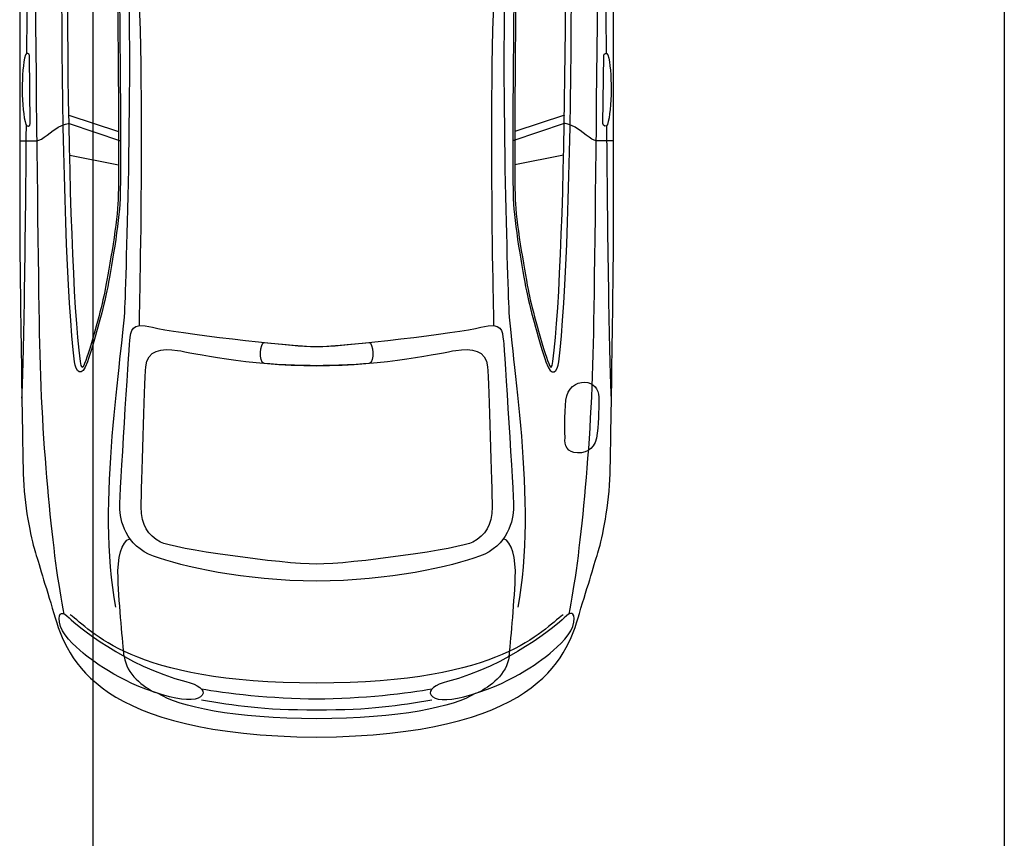
# Model space of a CAD drawing. Units: inches. Extents: x 1863 to 2938, y 1238 to 2492.
# Tile 3 of 12: x 2219 to 2283, y 1345 to 1398. Entities that reach past the tile are written whole.
import ezdxf

# ---------------------------------------------------------------- set-up
doc = ezdxf.new("R2010")
doc.units = ezdxf.units.IN
doc.layers.add('A-ANNO-DIMS', color=2, linetype='Continuous', lineweight=18)
doc.layers.add('AUDI', color=7, linetype='Continuous', lineweight=25)
doc.styles.get("Standard").update_dxf_attribs({"font": 'arial.ttf'})
doc.dimstyles.new('ISO-25', dxfattribs={"dimtxt": 7, "dimasz": 2.5, "dimexe": 1.25, "dimexo": 0.625, "dimtad": 1, "dimdec": 0, "dimlunit": 3, "dimtxsty": 'Standard', "dimcen": 2.5, "dimadec": 0, "dimazin": 0, "dimtfac": 1, "dimtdec": 0, "dimtmove": 0, "dimatfit": 3, "dimfxl": 1, "dimarcsym": 0})

# ---------------------------------------------------------------- blocks, each defined once
blk = doc.blocks.new('*D58')
at = {"layer": 'A-ANNO-DIMS', "color": 0, "lineweight": -2, "transparency": 16777216}
for p, q in [((2283.384, 1624.448), (2283.384, 1243.072)), ((2223.915, 1623.598), (2223.915, 1243.072)), ((2226.415, 1244.322), (2280.884, 1244.322))]:
    blk.add_line(p, q, dxfattribs=at)
at = {"layer": 'A-ANNO-DIMS', "color": 0, "transparency": 16777216}
for points in [[(2226.415, 1244.739), (2226.415, 1243.905), (2223.915, 1244.322)], [(2280.884, 1244.739), (2280.884, 1243.905), (2283.384, 1244.322)]]:
    blk.add_solid(points, dxfattribs=at)
at = {"layer": 'Defpoints', "color": 0, "transparency": 16777216}
for p in [(2283.384, 1625.073), (2223.915, 1624.223), (2283.384, 1244.322)]:
    blk.add_point(p, dxfattribs=at)
at = {"layer": 'A-ANNO-DIMS', "color": 0, "transparency": 16777216, "insert": (2253.65, 1248.566), "char_height": 7, "attachment_point": 5}
blk.add_mtext('4\'-11 1/2"', dxfattribs=at)

msp = doc.modelspace()

# ---------------------------------------------------------------- linework, layer by layer
at = {"layer": 'AUDI'}
for points, knots in [([(2238.512, 1351.601), (2224.304, 1351.757), (2222.24, 1356.535), (2221.369, 1359.683), (2221.369, 1359.683), (2220.8, 1361.542), (2220.345, 1363.021), (2220.118, 1363.779), (2220.118, 1363.779), (2219.89, 1364.538), (2219.398, 1366.852), (2219.359, 1368.786), (2219.359, 1368.786), (2219.321, 1370.721), (2219.134, 1382.255), (2219.134, 1385.438), (2219.134, 1385.438), (2219.134, 1388.621), (2219.134, 1403.534), (2219.134, 1405.655), (2219.134, 1405.655), (2219.134, 1407.776), (2219.587, 1416.238), (2219.587, 1418.931), (2219.587, 1418.931), (2219.587, 1421.624), (2219.134, 1425.003), (2219.134, 1426.403), (2219.134, 1426.403), (2219.134, 1427.803), (2219.397, 1435.203), (2219.511, 1436.834), (2219.511, 1436.834), (2219.625, 1438.465), (2220.236, 1439.39), (2220.762, 1440.551), (2220.762, 1440.551), (2222.809, 1445.064), (2228.041, 1447.53), (2228.61, 1447.909), (2228.61, 1447.909), (2229.178, 1448.289), (2229.782, 1448.495), (2230.505, 1448.495), (2230.505, 1448.495), (2231.228, 1448.495), (2231.415, 1448.137), (2231.718, 1448.213), (2231.718, 1448.213), (2232.021, 1448.289), (2232.777, 1448.495), (2233.614, 1448.495), (2233.614, 1448.495), (2234.451, 1448.495), (2238.512, 1448.495), (2238.512, 1448.495), (2238.512, 1448.495), (2238.512, 1448.495), (2242.574, 1448.495), (2243.411, 1448.495), (2243.411, 1448.495), (2244.248, 1448.495), (2245.003, 1448.289), (2245.306, 1448.213), (2245.306, 1448.213), (2245.61, 1448.137), (2245.796, 1448.495), (2246.52, 1448.495), (2246.52, 1448.495), (2247.243, 1448.495), (2247.846, 1448.289), (2248.415, 1447.909), (2248.415, 1447.909), (2248.984, 1447.53), (2254.215, 1445.064), (2256.262, 1440.551), (2256.262, 1440.551), (2256.789, 1439.39), (2257.4, 1438.465), (2257.513, 1436.834), (2257.513, 1436.834), (2257.627, 1435.203), (2257.891, 1427.803), (2257.891, 1426.403), (2257.891, 1426.403), (2257.891, 1425.003), (2257.438, 1421.624), (2257.438, 1418.931), (2257.438, 1418.931), (2257.438, 1416.238), (2257.891, 1407.776), (2257.891, 1405.655), (2257.891, 1405.655), (2257.891, 1403.534), (2257.891, 1388.621), (2257.891, 1385.438), (2257.891, 1385.438), (2257.891, 1382.255), (2257.703, 1370.721), (2257.665, 1368.786), (2257.665, 1368.786), (2257.627, 1366.852), (2257.134, 1364.538), (2256.907, 1363.779), (2256.907, 1363.779), (2256.679, 1363.021), (2256.225, 1361.541), (2255.656, 1359.683), (2255.656, 1359.683), (2254.784, 1356.535), (2252.721, 1351.757), (2238.512, 1351.601)], [0, 0, 0, 0, 0.035714, 0.035714, 0.035714, 0.035714, 0.071429, 0.071429, 0.071429, 0.071429, 0.107143, 0.107143, 0.107143, 0.107143, 0.142857, 0.142857, 0.142857, 0.142857, 0.178571, 0.178571, 0.178571, 0.178571, 0.214286, 0.214286, 0.214286, 0.214286, 0.25, 0.25, 0.25, 0.25, 0.285714, 0.285714, 0.285714, 0.285714, 0.321429, 0.321429, 0.321429, 0.321429, 0.357143, 0.357143, 0.357143, 0.357143, 0.392857, 0.392857, 0.392857, 0.392857, 0.428571, 0.428571, 0.428571, 0.428571, 0.464286, 0.464286, 0.464286, 0.464286, 0.5, 0.5, 0.5, 0.5, 0.535714, 0.535714, 0.535714, 0.535714, 0.571429, 0.571429, 0.571429, 0.571429, 0.607143, 0.607143, 0.607143, 0.607143, 0.642857, 0.642857, 0.642857, 0.642857, 0.678571, 0.678571, 0.678571, 0.678571, 0.714286, 0.714286, 0.714286, 0.714286, 0.75, 0.75, 0.75, 0.75, 0.785714, 0.785714, 0.785714, 0.785714, 0.821429, 0.821429, 0.821429, 0.821429, 0.857143, 0.857143, 0.857143, 0.857143, 0.892857, 0.892857, 0.892857, 0.892857, 0.928571, 0.928571, 0.928571, 0.928571, 0.964286, 0.964286, 0.964286, 0.964286, 1, 1, 1, 1]), ([(2222.035, 1359.641), (2221.321, 1363.213), (2220.561, 1370.446), (2220.431, 1377.979), (2220.431, 1377.979), (2220.301, 1385.512), (2219.977, 1414.474), (2220.172, 1420.578), (2220.172, 1420.578), (2220.366, 1426.682), (2220.475, 1434.382), (2221.557, 1439.624)], [0, 0, 0, 0, 0.333333, 0.333333, 0.333333, 0.333333, 0.666667, 0.666667, 0.666667, 0.666667, 1, 1, 1, 1]), ([(2254.99, 1359.641), (2255.704, 1363.213), (2256.464, 1370.446), (2256.593, 1377.979), (2256.593, 1377.979), (2256.723, 1385.512), (2257.048, 1414.474), (2256.853, 1420.578), (2256.853, 1420.578), (2256.658, 1426.682), (2256.549, 1434.382), (2255.468, 1439.624)], [0, 0, 0, 0, 0.333333, 0.333333, 0.333333, 0.333333, 0.666667, 0.666667, 0.666667, 0.666667, 1, 1, 1, 1]), ([(2222.717, 1376.103), (2222.793, 1375.509), (2223.16, 1374.97), (2223.554, 1376.103), (2223.554, 1376.103), (2223.947, 1377.235), (2224.587, 1379.549), (2224.784, 1380.534), (2224.784, 1380.534), (2224.981, 1381.519), (2225.572, 1384.768), (2225.67, 1386.393), (2225.67, 1386.393), (2225.768, 1388.018), (2225.67, 1396.339), (2225.67, 1398.308), (2225.67, 1398.308), (2225.67, 1400.278), (2224.833, 1407.024), (2224.538, 1408.648), (2224.538, 1408.648), (2224.243, 1410.273), (2223.603, 1413.523), (2222.371, 1417.183), (2222.371, 1417.183), (2221.635, 1413.129), (2221.733, 1383.833), (2222.717, 1376.103)], [0, 0, 0, 0, 0.142857, 0.142857, 0.142857, 0.142857, 0.285714, 0.285714, 0.285714, 0.285714, 0.428571, 0.428571, 0.428571, 0.428571, 0.571429, 0.571429, 0.571429, 0.571429, 0.714286, 0.714286, 0.714286, 0.714286, 0.857143, 0.857143, 0.857143, 0.857143, 1, 1, 1, 1]), ([(2254.308, 1376.103), (2254.232, 1375.509), (2253.864, 1374.97), (2253.471, 1376.103), (2253.471, 1376.103), (2253.077, 1377.235), (2252.437, 1379.549), (2252.241, 1380.534), (2252.241, 1380.534), (2252.044, 1381.519), (2251.453, 1384.768), (2251.355, 1386.393), (2251.355, 1386.393), (2251.256, 1388.018), (2251.355, 1396.339), (2251.355, 1398.308), (2251.355, 1398.308), (2251.355, 1400.278), (2252.191, 1407.024), (2252.487, 1408.648), (2252.487, 1408.648), (2252.782, 1410.273), (2253.422, 1413.523), (2254.654, 1417.183), (2254.654, 1417.183), (2255.39, 1413.129), (2255.292, 1383.833), (2254.308, 1376.103)], [0, 0, 0, 0, 0.142857, 0.142857, 0.142857, 0.142857, 0.285714, 0.285714, 0.285714, 0.285714, 0.428571, 0.428571, 0.428571, 0.428571, 0.571429, 0.571429, 0.571429, 0.571429, 0.714286, 0.714286, 0.714286, 0.714286, 0.857143, 0.857143, 0.857143, 0.857143, 1, 1, 1, 1]), ([(2223.091, 1376.134), (2223.091, 1376.134), (2223.091, 1376.134), (2223.091, 1376.134), (2223.091, 1376.134), (2223.119, 1375.917), (2223.178, 1375.791), (2223.221, 1375.73), (2223.221, 1375.73), (2223.266, 1375.783), (2223.344, 1375.902), (2223.442, 1376.185), (2223.442, 1376.185), (2223.826, 1377.289), (2224.465, 1379.591), (2224.663, 1380.583), (2224.663, 1380.583), (2224.901, 1381.772), (2225.453, 1384.89), (2225.545, 1386.408), (2225.545, 1386.408), (2225.617, 1387.597), (2225.582, 1392.452), (2225.559, 1395.665), (2225.559, 1395.665), (2225.559, 1395.665), (2225.544, 1398.309), (2225.544, 1398.309), (2225.544, 1398.309), (2225.544, 1400.273), (2224.699, 1407.05), (2224.417, 1408.603), (2224.417, 1408.603), (2223.944, 1411.2), (2223.332, 1413.673), (2222.608, 1415.993), (2222.608, 1415.993), (2222.029, 1409.274), (2222.179, 1383.297), (2223.091, 1376.134)], [0, 0, 0, 0, 0.1, 0.1, 0.1, 0.1, 0.2, 0.2, 0.2, 0.2, 0.3, 0.3, 0.3, 0.3, 0.4, 0.4, 0.4, 0.4, 0.5, 0.5, 0.5, 0.5, 0.6, 0.6, 0.6, 0.6, 0.7, 0.7, 0.7, 0.7, 0.8, 0.8, 0.8, 0.8, 0.9, 0.9, 0.9, 0.9, 1, 1, 1, 1]), ([(2253.933, 1376.134), (2253.933, 1376.134), (2253.933, 1376.134), (2253.933, 1376.134), (2253.933, 1376.134), (2253.906, 1375.917), (2253.846, 1375.791), (2253.804, 1375.73), (2253.804, 1375.73), (2253.759, 1375.783), (2253.681, 1375.902), (2253.582, 1376.185), (2253.582, 1376.185), (2253.199, 1377.289), (2252.56, 1379.591), (2252.361, 1380.583), (2252.361, 1380.583), (2252.124, 1381.772), (2251.572, 1384.89), (2251.48, 1386.408), (2251.48, 1386.408), (2251.408, 1387.597), (2251.442, 1392.452), (2251.465, 1395.665), (2251.465, 1395.665), (2251.465, 1395.665), (2251.48, 1398.309), (2251.48, 1398.309), (2251.48, 1398.309), (2251.48, 1400.273), (2252.326, 1407.05), (2252.608, 1408.603), (2252.608, 1408.603), (2253.08, 1411.2), (2253.692, 1413.673), (2254.417, 1415.993), (2254.417, 1415.993), (2254.995, 1409.274), (2254.846, 1383.297), (2253.933, 1376.134)], [0, 0, 0, 0, 0.1, 0.1, 0.1, 0.1, 0.2, 0.2, 0.2, 0.2, 0.3, 0.3, 0.3, 0.3, 0.4, 0.4, 0.4, 0.4, 0.5, 0.5, 0.5, 0.5, 0.6, 0.6, 0.6, 0.6, 0.7, 0.7, 0.7, 0.7, 0.8, 0.8, 0.8, 0.8, 0.9, 0.9, 0.9, 0.9, 1, 1, 1, 1]), ([(2226.062, 1406.214), (2226.571, 1397.024), (2226.092, 1382.572), (2225.981, 1379.639), (2225.981, 1379.639), (2225.87, 1376.706), (2224.075, 1366.744), (2225.391, 1360.079)], [0, 0, 0, 0, 0.5, 0.5, 0.5, 0.5, 1, 1, 1, 1]), ([(2250.963, 1406.214), (2250.454, 1397.024), (2250.933, 1382.572), (2251.044, 1379.639), (2251.044, 1379.639), (2251.154, 1376.706), (2252.949, 1366.744), (2251.634, 1360.079)], [0, 0, 0, 0, 0.5, 0.5, 0.5, 0.5, 1, 1, 1, 1]), ([(2219.828, 1391.652), (2219.828, 1391.478), (2219.591, 1391.413), (2219.538, 1391.587), (2219.538, 1391.587), (2219.379, 1392.086), (2219.301, 1392.976), (2219.301, 1393.866), (2219.301, 1393.866), (2219.301, 1394.757), (2219.353, 1395.625), (2219.511, 1396.146), (2219.511, 1396.146), (2219.564, 1396.298), (2219.775, 1396.255), (2219.775, 1396.081), (2219.775, 1396.081), (2219.775, 1396.081), (2219.828, 1391.652), (2219.828, 1391.652)], [0, 0, 0, 0, 0.2, 0.2, 0.2, 0.2, 0.4, 0.4, 0.4, 0.4, 0.6, 0.6, 0.6, 0.6, 0.8, 0.8, 0.8, 0.8, 1, 1, 1, 1]), ([(2257.196, 1391.652), (2257.196, 1391.478), (2257.434, 1391.413), (2257.487, 1391.587), (2257.487, 1391.587), (2257.645, 1392.086), (2257.724, 1392.976), (2257.724, 1393.866), (2257.724, 1393.866), (2257.724, 1394.757), (2257.671, 1395.625), (2257.513, 1396.146), (2257.513, 1396.146), (2257.46, 1396.298), (2257.25, 1396.255), (2257.25, 1396.081), (2257.25, 1396.081), (2257.25, 1396.081), (2257.196, 1391.652), (2257.196, 1391.652)], [0, 0, 0, 0, 0.2, 0.2, 0.2, 0.2, 0.4, 0.4, 0.4, 0.4, 0.6, 0.6, 0.6, 0.6, 0.8, 0.8, 0.8, 0.8, 1, 1, 1, 1]), ([(2219.134, 1390.537), (2219.134, 1390.537), (2219.988, 1390.537), (2220.268, 1390.537), (2220.268, 1390.537), (2220.548, 1390.537), (2221.292, 1391.217), (2221.635, 1391.415), (2221.635, 1391.415), (2221.977, 1391.614), (2222.354, 1391.661), (2222.354, 1391.661)], [0, 0, 0, 0, 0.333333, 0.333333, 0.333333, 0.333333, 0.666667, 0.666667, 0.666667, 0.666667, 1, 1, 1, 1]), ([(2257.891, 1390.537), (2257.891, 1390.537), (2257.037, 1390.537), (2256.757, 1390.537), (2256.757, 1390.537), (2256.476, 1390.537), (2255.733, 1391.217), (2255.39, 1391.415), (2255.39, 1391.415), (2255.047, 1391.614), (2254.671, 1391.661), (2254.671, 1391.661)], [0, 0, 0, 0, 0.333333, 0.333333, 0.333333, 0.333333, 0.666667, 0.666667, 0.666667, 0.666667, 1, 1, 1, 1]), ([(2238.512, 1361.794), (2243.289, 1361.794), (2247.305, 1362.753), (2249.149, 1363.417), (2249.149, 1363.417), (2250.992, 1364.081), (2251.361, 1365.778), (2251.361, 1366.627), (2251.361, 1366.627), (2251.361, 1367.475), (2250.771, 1376.809), (2250.697, 1377.473), (2250.697, 1377.473), (2250.624, 1378.137), (2250.66, 1378.728), (2249.222, 1378.359), (2249.222, 1378.359), (2247.784, 1377.99), (2240.299, 1377.104), (2238.512, 1377.104), (2238.512, 1377.104), (2236.726, 1377.105), (2229.24, 1377.99), (2227.802, 1378.359), (2227.802, 1378.359), (2226.364, 1378.728), (2226.401, 1378.137), (2226.327, 1377.473), (2226.327, 1377.473), (2226.254, 1376.809), (2225.664, 1367.475), (2225.664, 1366.627), (2225.664, 1366.627), (2225.664, 1365.778), (2226.032, 1364.081), (2227.876, 1363.417), (2227.876, 1363.417), (2229.72, 1362.753), (2233.735, 1361.794), (2238.512, 1361.794)], [0, 0, 0, 0, 0.1, 0.1, 0.1, 0.1, 0.2, 0.2, 0.2, 0.2, 0.3, 0.3, 0.3, 0.3, 0.4, 0.4, 0.4, 0.4, 0.5, 0.5, 0.5, 0.5, 0.6, 0.6, 0.6, 0.6, 0.7, 0.7, 0.7, 0.7, 0.8, 0.8, 0.8, 0.8, 0.9, 0.9, 0.9, 0.9, 1, 1, 1, 1]), ([(2238.512, 1361.794), (2243.289, 1361.794), (2247.305, 1362.753), (2249.149, 1363.417), (2249.149, 1363.417), (2250.992, 1364.081), (2251.361, 1365.778), (2251.361, 1366.627), (2251.361, 1366.627), (2251.361, 1367.475), (2250.771, 1376.809), (2250.697, 1377.473), (2250.697, 1377.473), (2250.624, 1378.137), (2250.66, 1378.728), (2249.222, 1378.359), (2249.222, 1378.359), (2247.784, 1377.99), (2240.299, 1377.104), (2238.512, 1377.104), (2238.512, 1377.104), (2236.726, 1377.104), (2229.24, 1377.99), (2227.802, 1378.359), (2227.802, 1378.359), (2226.364, 1378.728), (2226.401, 1378.137), (2226.327, 1377.473), (2226.327, 1377.473), (2226.254, 1376.809), (2225.664, 1367.475), (2225.664, 1366.627), (2225.664, 1366.627), (2225.664, 1365.778), (2226.032, 1364.081), (2227.876, 1363.417), (2227.876, 1363.417), (2229.72, 1362.753), (2233.735, 1361.794), (2238.512, 1361.794)], [0, 0, 0, 0, 0.1, 0.1, 0.1, 0.1, 0.2, 0.2, 0.2, 0.2, 0.3, 0.3, 0.3, 0.3, 0.4, 0.4, 0.4, 0.4, 0.5, 0.5, 0.5, 0.5, 0.6, 0.6, 0.6, 0.6, 0.7, 0.7, 0.7, 0.7, 0.8, 0.8, 0.8, 0.8, 0.9, 0.9, 0.9, 0.9, 1, 1, 1, 1]), ([(2238.512, 1362.898), (2240.778, 1362.898), (2247.895, 1363.897), (2248.706, 1364.339), (2248.706, 1364.339), (2249.517, 1364.782), (2249.96, 1365.409), (2249.96, 1366.627), (2249.96, 1366.627), (2249.96, 1367.844), (2249.738, 1374.67), (2249.665, 1375.776), (2249.665, 1375.776), (2249.591, 1376.883), (2248.595, 1376.994), (2247.6, 1376.846), (2247.6, 1376.846), (2246.604, 1376.699), (2243.101, 1375.85), (2238.512, 1375.85), (2238.512, 1375.85), (2233.923, 1375.85), (2230.42, 1376.699), (2229.425, 1376.846), (2229.425, 1376.846), (2228.429, 1376.994), (2227.434, 1376.883), (2227.36, 1375.776), (2227.36, 1375.776), (2227.286, 1374.67), (2227.065, 1367.844), (2227.065, 1366.627), (2227.065, 1366.627), (2227.065, 1365.409), (2227.507, 1364.782), (2228.318, 1364.339), (2228.318, 1364.339), (2229.13, 1363.897), (2236.246, 1362.898), (2238.512, 1362.898)], [0, 0, 0, 0, 0.1, 0.1, 0.1, 0.1, 0.2, 0.2, 0.2, 0.2, 0.3, 0.3, 0.3, 0.3, 0.4, 0.4, 0.4, 0.4, 0.5, 0.5, 0.5, 0.5, 0.6, 0.6, 0.6, 0.6, 0.7, 0.7, 0.7, 0.7, 0.8, 0.8, 0.8, 0.8, 0.9, 0.9, 0.9, 0.9, 1, 1, 1, 1]), ([(2238.512, 1375.85), (2238.512, 1375.85), (2241.218, 1375.898), (2241.924, 1376.002), (2241.924, 1376.002), (2242.365, 1376.067), (2242.157, 1377.387), (2241.951, 1377.367), (2241.951, 1377.367), (2240.654, 1377.241), (2239.564, 1377.104), (2238.512, 1377.104), (2238.512, 1377.104), (2237.46, 1377.104), (2236.37, 1377.241), (2235.074, 1377.367), (2235.074, 1377.367), (2234.867, 1377.387), (2234.66, 1376.067), (2235.101, 1376.002), (2235.101, 1376.002), (2235.807, 1375.898), (2238.512, 1375.85), (2238.512, 1375.85)], [0, 0, 0, 0, 0.166667, 0.166667, 0.166667, 0.166667, 0.333333, 0.333333, 0.333333, 0.333333, 0.5, 0.5, 0.5, 0.5, 0.666667, 0.666667, 0.666667, 0.666667, 0.833333, 0.833333, 0.833333, 0.833333, 1, 1, 1, 1]), ([(2254.721, 1371.148), (2254.669, 1370.666), (2254.842, 1370.166), (2255.542, 1370.152), (2255.542, 1370.152), (2256.241, 1370.139), (2256.722, 1370.512), (2256.824, 1371.436), (2256.824, 1371.436), (2256.927, 1372.36), (2256.927, 1373.284), (2256.927, 1373.797), (2256.927, 1373.797), (2256.927, 1374.31), (2256.568, 1374.772), (2256.003, 1374.772), (2256.003, 1374.772), (2255.439, 1374.772), (2254.875, 1374.413), (2254.772, 1373.592), (2254.772, 1373.592), (2254.669, 1372.77), (2254.721, 1371.148), (2254.721, 1371.148)], [0, 0, 0, 0, 0.166667, 0.166667, 0.166667, 0.166667, 0.333333, 0.333333, 0.333333, 0.333333, 0.5, 0.5, 0.5, 0.5, 0.666667, 0.666667, 0.666667, 0.666667, 0.833333, 0.833333, 0.833333, 0.833333, 1, 1, 1, 1]), ([(2225.959, 1356.873), (2225.85, 1357.783), (2225.635, 1360.112), (2225.553, 1361.997), (2225.553, 1361.997), (2225.498, 1363.269), (2225.771, 1364.404), (2226.326, 1364.556)], [0, 0, 0, 0, 0.5, 0.5, 0.5, 0.5, 1, 1, 1, 1]), ([(2251.065, 1356.873), (2251.174, 1357.783), (2251.39, 1360.112), (2251.472, 1361.997), (2251.472, 1361.997), (2251.527, 1363.269), (2251.254, 1364.404), (2250.699, 1364.556)], [0, 0, 0, 0, 0.5, 0.5, 0.5, 0.5, 1, 1, 1, 1]), ([(2229.983, 1355.232), (2226.043, 1356.251), (2222.853, 1358.906), (2222.361, 1359.384), (2222.361, 1359.384), (2221.928, 1359.804), (2221.662, 1359.85), (2221.729, 1359.11), (2221.729, 1359.11), (2221.796, 1358.379), (2222.717, 1357.556), (2223.283, 1357.087), (2223.283, 1357.087), (2224.005, 1356.487), (2225.988, 1354.992), (2228.917, 1354.246), (2228.917, 1354.246), (2230.036, 1353.926), (2230.835, 1354.033), (2231.048, 1354.352), (2231.048, 1354.352), (2231.261, 1354.672), (2230.765, 1355.028), (2229.983, 1355.232)], [0, 0, 0, 0, 0.166667, 0.166667, 0.166667, 0.166667, 0.333333, 0.333333, 0.333333, 0.333333, 0.5, 0.5, 0.5, 0.5, 0.666667, 0.666667, 0.666667, 0.666667, 0.833333, 0.833333, 0.833333, 0.833333, 1, 1, 1, 1]), ([(2254.596, 1359.588), (2253.186, 1358.621), (2250.775, 1355.134), (2238.512, 1355.134), (2238.512, 1355.134), (2226.25, 1355.134), (2223.838, 1358.621), (2222.429, 1359.588)], [0, 0, 0, 0, 0.5, 0.5, 0.5, 0.5, 1, 1, 1, 1]), ([(2247.042, 1355.232), (2250.981, 1356.251), (2254.172, 1358.906), (2254.664, 1359.384), (2254.664, 1359.384), (2255.097, 1359.804), (2255.363, 1359.85), (2255.295, 1359.11), (2255.295, 1359.11), (2255.228, 1358.379), (2254.307, 1357.556), (2253.742, 1357.087), (2253.742, 1357.087), (2253.019, 1356.487), (2251.037, 1354.992), (2248.107, 1354.246), (2248.107, 1354.246), (2246.989, 1353.926), (2246.19, 1354.033), (2245.977, 1354.352), (2245.977, 1354.352), (2245.764, 1354.672), (2246.26, 1355.028), (2247.042, 1355.232)], [0, 0, 0, 0, 0.166667, 0.166667, 0.166667, 0.166667, 0.333333, 0.333333, 0.333333, 0.333333, 0.5, 0.5, 0.5, 0.5, 0.666667, 0.666667, 0.666667, 0.666667, 0.833333, 0.833333, 0.833333, 0.833333, 1, 1, 1, 1]), ([(2248.858, 1354.459), (2247.489, 1353.585), (2243.916, 1352.81), (2238.512, 1352.81), (2238.512, 1352.81), (2233.108, 1352.81), (2229.535, 1353.585), (2228.166, 1354.459)], [0, 0, 0, 0, 0.5, 0.5, 0.5, 0.5, 1, 1, 1, 1]), ([(2246.036, 1354.741), (2244.613, 1354.47), (2241.372, 1354.083), (2238.512, 1354.083), (2238.512, 1354.083), (2235.653, 1354.083), (2232.411, 1354.47), (2230.989, 1354.741)], [0, 0, 0, 0, 0.5, 0.5, 0.5, 0.5, 1, 1, 1, 1]), ([(2246.036, 1354.028), (2243.839, 1353.641), (2242.091, 1353.364), (2238.512, 1353.364), (2238.512, 1353.364), (2234.934, 1353.364), (2233.186, 1353.641), (2230.989, 1354.028)], [0, 0, 0, 0, 0.5, 0.5, 0.5, 0.5, 1, 1, 1, 1])]:
    msp.add_open_spline(points, degree=3, knots=knots, dxfattribs=at)
for points in [[(2219.604, 1396.234), (2219.653, 1405.036), (2219.647, 1413.789), (2219.558, 1417.313)], [(2257.421, 1396.234), (2257.372, 1405.036), (2257.378, 1413.789), (2257.467, 1417.313)], [(2226.942, 1378.466), (2226.942, 1378.466), (2227.414, 1397.291), (2226.631, 1405.331)], [(2250.082, 1378.466), (2250.082, 1378.466), (2249.61, 1397.291), (2250.394, 1405.331)], [(2222.345, 1392.198), (2222.345, 1392.198), (2225.586, 1391.134), (2225.586, 1391.134)], [(2254.68, 1392.198), (2254.68, 1392.198), (2251.439, 1391.134), (2251.439, 1391.134)], [(2219.277, 1373.726), (2219.403, 1375.974), (2219.51, 1383.358), (2219.573, 1391.525)], [(2222.354, 1391.661), (2222.354, 1391.661), (2225.713, 1390.537), (2225.713, 1390.537)], [(2254.671, 1391.661), (2254.671, 1391.661), (2251.312, 1390.537), (2251.312, 1390.537)], [(2257.748, 1373.726), (2257.622, 1375.974), (2257.515, 1383.358), (2257.452, 1391.525)], [(2222.397, 1389.591), (2222.397, 1389.591), (2225.587, 1388.953), (2225.587, 1388.953)], [(2254.628, 1389.591), (2254.628, 1389.591), (2251.438, 1388.953), (2251.438, 1388.953)], [(2225.959, 1356.873), (2226.083, 1355.707), (2227.227, 1354.876), (2227.97, 1354.522)], [(2251.065, 1356.873), (2250.941, 1355.707), (2249.798, 1354.876), (2249.054, 1354.522)]]:
    msp.add_open_spline(points, degree=3, dxfattribs=at)

# ---------------------------------------------------------------- dimensions: what is measured, and where the dimension line sits
at = {"layer": 'A-ANNO-DIMS'}
dim = msp.add_linear_dim(base=(2283.384, 1244.322), p1=(2223.915, 1624.223), p2=(2283.384, 1625.073), dimstyle='ISO-25', override={"dimdec": 1, "dimlfac": 1, "dimrnd": 0, "dimzin": 1, "dimdsep": 46, "dimlunit": 4, "dimfrac": 2}, dxfattribs=at)
dim.commit()
dim.dimension.update_dxf_attribs({"geometry": '*D58', "text_midpoint": (2253.65, 1248.566)})

doc.saveas('drawing.dxf')
